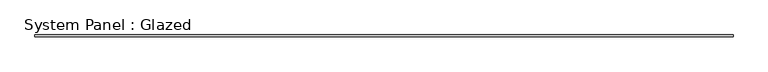
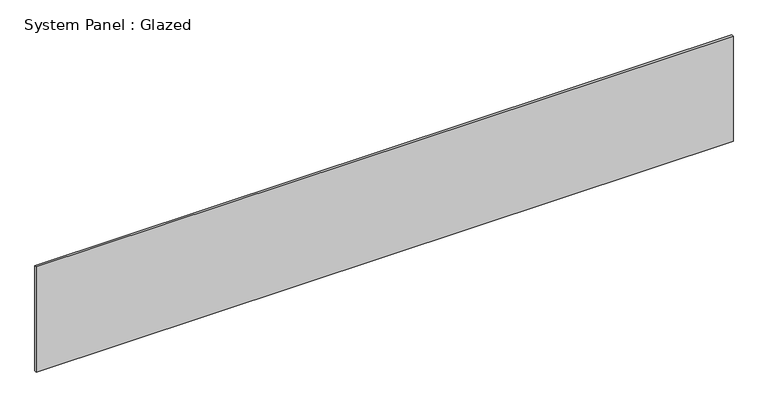
"""IFC4 building model written with IfcOpenShell, lengths in millimetres: plate geometry, System Panel : Glazed."""

from ifc_helpers import new_model, si_unit, origin, origin_with_axes, place, context, project, spatial, polyline, outline, extrude, source, transform, mapped, element, save


def system_panel_glazed_1fde7296(model_context):
    return source(origin(), model_context, "Body", "SweptSolid", [
        extrude(outline(polyline([(4578.35, 19.05), (-4578.35, 19.05), (-4578.35, 44.45), (4578.35, 44.45), (4578.35, 19.05)])), origin_with_axes(), (0.0, 0.0, 1.0), 1460.5),
    ])


if __name__ == "__main__":
    model = new_model("IFC4")
    model_context = context("Model", 3, world=origin())
    ifc_project = project(units=[si_unit("LENGTHUNIT", "METRE", prefix="MILLI")], contexts=[model_context])
    site = spatial("IfcSite", under=ifc_project)
    building = spatial("IfcBuilding", under=site)
    placement = place(None, origin())
    system_panel_glazed_shape = system_panel_glazed_1fde7296(model_context)
    element("IfcPlate", 1, ObjectType="System Panel : Glazed", at=placement, inside=building, context=model_context, shape_type="MappedRepresentation", body=[
        mapped(system_panel_glazed_shape, transform((0.0, 0.0, 0.0), x_axis=(1.0, 0.0, 0.0), y_axis=(0.0, 1.0, 0.0), z_axis=(0.0, 0.0, 1.0))),
    ])
    save(model, "model.ifc")

# Revit data of these elements
# Type "System Panel : Glazed"
#   Construction Type Id = "GSP4R"
#   Analytic Construction = "1/8 in Pilkington single glazing"
#   Visual Light Transmittance = 0.9
#   Solar Heat Gain Coefficient = 0.86
#   Heat Transfer Coefficient (U) = 1.18115 BTU/(h·ft²·°F)
# Element 1 (IfcPlate, "System Panel : Glazed")
#   Materials on its faces: "Glass"
# Materials
#   "Glass": class "Glass", colour RGB 0 128 192, transparency 0.75, Description = "Soda Lime Glass", Cost = 0
